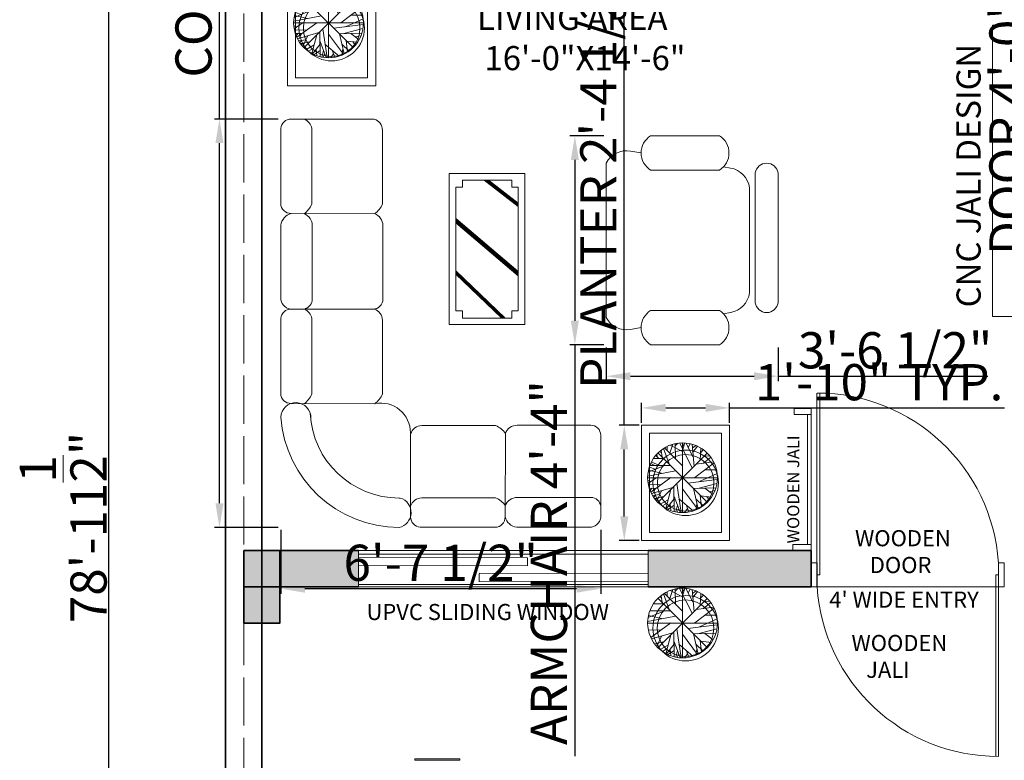
# Model space of a CAD drawing. Units: millimetres. Extents: x 595116 to 630915, y 909473 to 920225.
# Tile 118 of 134: x 629260 to 629505, y 919558 to 919742. Entities that reach past the tile are written whole.
import ezdxf

# ---------------------------------------------------------------- set-up
doc = ezdxf.new("R2010")
doc.units = ezdxf.units.MM
doc.linetypes.add('ACAD_ISO02W100', pattern=[15, 12, -3])
for name, color, linetype, lineweight in [('A-AREA-IDEN', 7, 'Continuous', 20), ('A-FLOR-SCRN', 31, 'Continuous', 18), ('A-FURN', 32, 'Continuous', 18), ('A-WALL', 1, 'Continuous', 35), ('A-WALL-PATT', 8, 'Continuous', 13), ('C-PRKG-VEHI', 8, 'Continuous', 13), ('C-PROP-REF', 240, 'ACAD_ISO02W100', 13), ('Column', 6, 'Continuous', 35), ('Dimension', 3, 'Continuous', 18), ('Doors', 31, 'Continuous', 20), ('L-PLNT', 85, 'Continuous', 13), ('Text', 7, 'Continuous', 18), ('Windows', 33, 'Continuous', 18)]:
    doc.layers.add(name, color=color, linetype=linetype, lineweight=lineweight)
doc.styles.get("Standard").update_dxf_attribs({"font": 'arial.ttf'})
doc.dimstyles.new('ISO-25', dxfattribs={"dimtxt": 9, "dimasz": 6, "dimexe": 1.25, "dimexo": 0.625, "dimtad": 1, "dimlunit": 4, "dimtxsty": 'Standard', "dimcen": 2.5, "dimadec": 0, "dimazin": 0, "dimtfac": 1, "dimtmove": 0, "dimatfit": 3, "dimfxl": 1, "dimarcsym": 0})

# ---------------------------------------------------------------- blocks, each defined once
blk = doc.blocks.new('KWD')
for points in [[(629753.63, 919957.93), (629752.54, 919957.93), (629752.54, 919953.43), (629753.63, 919953.43)], [(629787.45, 919957.93), (629787.45, 919953.43), (629788.54, 919953.43), (629788.54, 919957.93)]]:
    blk.add_lwpolyline(points, close=True)
blk.add_lwpolyline([(629753.63, 919921.79), (629753.63, 919955.68), (629754.13, 919955.68), (629754.13, 919921.8)])
blk.add_arc((629753.64, 919955.68), 33.88, 269.99, 356.196)
blk = doc.blocks.new('A$C2F471D6A')
for p, q in [((2695.9, 2657.3), (2692.2, 1939.9)), ((1797.2, 841.3), (2182.6, 1242.6)), ((1797.2, 833.9), (2189.8, 1242.6)), ((1797.2, 826.4), (2197, 1242.6)), ((1797.2, 818.9), (2204.2, 1242.6)), ((1797.2, 848.8), (2175.4, 1242.6)), ((2161.4, 709.9), (2615.3, 1243.3)), ((2168.6, 709.9), (2622.5, 1243.3)), ((2175.8, 709.9), (2629.7, 1243.3)), ((2183, 709.9), (2636.9, 1243.3)), ((2190.2, 709.9), (2644.1, 1243.3)), ((2197.4, 709.9), (2651.3, 1243.3)), ((2755.3, 709.9), (2980.5, 1000.5)), ((2762.5, 709.9), (2981.1, 992)), ((2769.7, 709.9), (2981.1, 982.7)), ((2776.9, 709.9), (2981.1, 973.4)), ((2784.1, 709.9), (2981.1, 964.1)), ((807.3, 817.6), (89.9, 821.3))]:
    blk.add_line(p, q)
for points in [[(0, 1730, -0.393715), (947.4, 2744.8)], [(946.9, 2744.9, -1), (937.9, 2487, 1)], [(1060.8, 1939.9, 0.132391), (1145.9, 1873.4), (1778.5, 1873.4, 0.326313), (1874.7, 1943.6), (1874.7, 2657.3, 0.389129), (1793.3, 2746), (1149.6, 2746, 0.426582), (1064.5, 2657.3, 0.287811)], [(1060.8, 2545.7, 0.132391), (1145.9, 2479.2), (1778.5, 2479.2, 0.287096), (1869.3, 2536)], [(1878.2, 2536, 0.331063), (1959.6, 2475.5), (2433.2, 2475.5)], [(2433.2, 2475.5), (2592.3, 2475.5, 0.316456), (2692.2, 2545.7, 0.132391), (2777.2, 2479.2), (3409.9, 2479.2, 0.287096), (3500.7, 2536)], [(252.5, 1720.4), (252.5, 1729.1, -0.399385), (979.3, 2493.9)], [(812.9, 1633.4, 0.469502), (1063.7, 1935.5, -1.204519)], [(252.5, 1720.4, -0.77294), (0, 1730, -1)], [(257.4, 558.6), (257.4, 717.7, 0.316456), (187.2, 817.6, 0.132391), (253.7, 902.7), (253.7, 1535.3, 0.326313), (183.5, 1631.5), (180.9, 1631.5, 0.389129)], [(180.9, 0.4, 0.385191), (257.4, 85.1), (257.4, 558.6)]]:
    blk.add_lwpolyline(points, format="xyb")
for points in [[(2433.2, 1869.7), (2592.3, 1869.7, 0.316456), (2692.2, 1939.9, 0.132391), (2777.2, 1873.4), (3409.9, 1873.4, 0.326313), (3506.1, 1943.6), (3506.1, 2657.3, 0.389129), (3424.7, 2746), (2780.9, 2746, 0.426582), (2695.9, 2657.3, 0.287811), (2596, 2746), (1970.7, 2746, 0.366167), (1874.5, 2664.7), (1874.5, 1954.7, 0.414362), (1959.6, 1869.7)], [(877.5, 558.6), (877.5, 717.7, 0.316456), (807.3, 817.6, 0.132391), (873.8, 902.7), (873.8, 1535.3, 0.326313), (803.6, 1631.5), (89.9, 1631.5, 0.389129), (1.2, 1550.1), (1.2, 906.4, 0.426582), (89.9, 821.3, 0.287811), (1.2, 721.4), (1.2, 96.2, 0.366167), (82.5, 0), (792.5, 0, 0.414362), (877.5, 85.1)]]:
    blk.add_lwpolyline(points, format="xyb", close=True)
blk.add_lwpolyline([(1064.5, 2657.3), (1060.8, 1939.9)])
for points in [[(1742.1, 652.3), (1742.1, 1300.3), (3038.1, 1300.3), (3038.1, 652.3)], [(2981.1, 1185.5), (2920, 1185.5), (2920, 1242.6), (1860.2, 1242.6), (1860.2, 1185.5), (1797.2, 1185.5), (1797.2, 762.2), (1860.2, 762.2), (1860.2, 709.1), (2920, 709.1), (2920, 762.2), (2981.1, 762.2)]]:
    blk.add_lwpolyline(points, close=True)
blk = doc.blocks.new('A$C20666D62')
for p, q in [((444.1, 457.2), (99.1, 457.2)), ((444.1, 396.2), (99.1, 396.2)), ((418, 381), (138.3, 381)), ((82.7, 311.8), (86, 330.2)), ((473.6, 311.8), (470.3, 330.2)), ((0, 118.1), (0, 301)), ((91.4, 301), (91.4, 118.1)), ((464.9, 301), (464.9, 118.1)), ((556.2, 118.1), (556.2, 301)), ((45.7, 92.8), (41.2, 64.6)), ((510.5, 92.8), (515.1, 64.6)), ((72.9, 0), (483.4, 0))]:
    blk.add_line(p, q)
for centre, radius, start, end in [((103.7, 426.7), 30.8, 98.7722, 261.228), ((439.5, 426.7), 30.8, 278.771, 81.2286), ((146.7, 320), 61.6, 97.9219, 170.441), ((409.6, 320), 61.6, 9.5598, 82.0778), ((45.7, 272.6), 53.9, 31.8953, 148.105), ((510.5, 272.6), 53.9, 31.8953, 148.105), ((45.7, 146.6), 53.8, 211.888, 328.112), ((510.5, 146.6), 53.8, 211.888, 328.112), ((98.9, 52.9), 58.9, 168.447, 243.852), ((457.4, 52.9), 58.9, 296.148, 11.5527)]:
    blk.add_arc(centre, radius, start, end)
blk = doc.blocks.new('A$C7ADB3080')
for p, q in [((0, 1141.1), (0, 1143.7)), ((0, 1143.7), (10.2, 1143.5)), ((0, 1136.6), (0, 1141.1)), ((0, 1131), (0, 1136.6)), ((0, 821.3), (0, 1131)), ((10.2, 1143.5), (10.2, 1140.7)), ((10.2, 1140.9), (10.2, 1143.5)), ((10.2, 1136.4), (10.2, 1140.9)), ((10.2, 1140.7), (10.2, 1136)), ((10.2, 1131.1), (10.2, 1136.4)), ((10.2, 1136), (10.2, 1130.9)), ((10.2, 821.4), (10.2, 1131.1)), ((10.2, 1130.9), (10.2, 821.4)), ((0, 816.5), (0, 821.3)), ((0, 812), (0, 816.5)), ((0, 808.8), (0, 812)), ((0, 808.8), (10.2, 808.8)), ((0, 808.8), (10.2, 808.7)), ((10.2, 816.5), (10.2, 821.4)), ((10.2, 821.4), (10.2, 816)), ((10.2, 811.8), (10.2, 816.5)), ((10.2, 816), (10.2, 811.6)), ((10.2, 808.8), (10.2, 811.8)), ((10.2, 811.6), (10.2, 808.7)), ((10.2, 808.7), (10.2, 808.8))]:
    blk.add_line(p, q)
blk = doc.blocks.new('*D128')
at = {"layer": 'Defpoints', "color": 0, "transparency": 16777216}
for p in [(629311.54, 920089.43), (629282.4, 919141.93), (629311.54, 919141.93)]:
    blk.add_point(p, dxfattribs=at)
at = {"layer": 'Dimension', "color": 0, "lineweight": -2, "transparency": 16777216}
for p, q in [((629310.92, 920089.43), (629281.15, 920089.43)), ((629282.4, 920083.43), (629282.4, 919147.93)), ((629310.92, 919141.93), (629281.15, 919141.93))]:
    blk.add_line(p, q, dxfattribs=at)
at = {"layer": 'Dimension', "color": 0, "transparency": 16777216}
for points in [[(629281.4, 920083.43), (629283.4, 920083.43), (629282.4, 920089.43)], [(629281.4, 919147.93), (629283.4, 919147.93), (629282.4, 919141.93)]]:
    blk.add_solid(points, dxfattribs=at)
at = {"layer": 'Dimension', "color": 0, "transparency": 16777216, "insert": (629271.16, 919615.68), "char_height": 9, "attachment_point": 5, "rotation": 90}
blk.add_mtext('78\'-11{\\H1x;\\S1/2;}"', dxfattribs=at)
blk = doc.blocks.new('POTTED-PLANT')
for p, q in [((4.85, 16.17), (4.88, 17.22)), ((5.49, 15.52), (6.28, 17.77)), ((5.61, 17.51), (8.67, 15.94)), ((6.86, 17.38), (7.52, 18.03)), ((6.89, 14.08), (6.86, 17.93)), ((7.9, 18.06), (11.06, 11.86)), ((9.02, 17.38), (8.46, 18.1)), ((8.67, 18.11), (8.67, 0.76)), ((8.74, 16.47), (9.2, 18.06)), ((11.32, 14.57), (9.46, 18.06)), ((10.09, 16.89), (10.53, 17.9)), ((11.52, 12.26), (11.04, 17.77)), ((11.14, 16.82), (12.03, 17.41)), ((11.24, 15.75), (12.36, 17.28)), ((14.75, 15.51), (2.6, 3.36)), ((14.75, 3.36), (2.6, 15.51)), ((2.87, 15.88), (3.4, 15.68)), ((3.32, 16.24), (3.58, 14.57)), ((3.96, 16.73), (5.31, 12.84)), ((4.16, 16.82), (8.64, 12.35)), ((13.25, 16.79), (13.05, 13.86)), ((13.17, 15.58), (13.86, 16.4)), ((14.04, 14.8), (15.41, 14.87)), ((4.01, 12.42), (0.12, 10.79)), ((0.57, 12.45), (5.66, 12.45)), ((1.47, 14.18), (3.93, 14.18)), ((16.53, 13.1), (11.7, 9.48)), ((12.05, 12.81), (16.38, 13.4)), ((13.91, 13.07), (15.74, 14.51)), ((0.04, 9.84), (6.94, 11.18)), ((0.19, 11.28), (3.48, 10.53)), ((12.92, 8.47), (17.27, 10.46)), ((14.24, 11.38), (17.09, 11.41)), ((0, 9.44), (17.35, 9.44)), ((0.22, 7.66), (3.4, 7.75)), ((0.78, 5.86), (5.74, 9.45)), ((7.22, 7.98), (8.31, 0.8)), ((10.02, 8.11), (17.3, 9.03)), ((12.49, 6.77), (17.19, 8.01)), ((0.98, 5.47), (6.25, 7.04)), ((3.48, 6.19), (2.31, 3.58)), ((5.79, 6.51), (4.54, 1.82)), ((6.53, 7.26), (6.56, 1.1)), ((8.67, 6.68), (12.41, 1.65)), ((11.37, 6.74), (12.54, 1.72)), ((11.39, 6.74), (16.97, 6.94)), ((13.07, 5.08), (13.35, 2.21)), ((13.22, 4.91), (15.85, 4.62)), ((14.19, 6.81), (16.25, 5.24)), ((3.99, 4.75), (1.72, 4.29)), ((5.1, 3.97), (3.07, 2.83)), ((4.88, 3.09), (3.65, 2.4)), ((6.56, 4.2), (4.67, 1.78)), ((6.56, 2.6), (5.05, 1.59)), ((5.56, 2.86), (5.79, 1.33)), ((6.56, 4.78), (8.11, 0.84)), ((7.45, 2.57), (7.01, 0.97)), ((7.78, 4.2), (11.26, 1.2)), ((9.53, 2.7), (10.2, 0.97)), ((11.98, 4.16), (13.78, 2.43)), ((12.26, 2.96), (12, 1.49)), ((7.75, 1.82), (7.32, 0.93)), ((9.89, 1.75), (9.23, 0.84))]:
    blk.add_line(p, q)
for centre, radius in [((8.67, 9.44), 8.67), ((9.43, 8.14), 8.14), ((9.43, 8.14), 7.03)]:
    blk.add_circle(centre, radius)
blk = doc.blocks.new('PLANTER-RECT')
for p, q in [((4.38, 22.08), (4.91, 21.89)), ((4.83, 22.44), (5.09, 20.78)), ((5.47, 22.93), (6.82, 19.05)), ((5.67, 23.03), (10.15, 18.56)), ((6.36, 22.38), (6.39, 23.42)), ((7, 21.72), (7.79, 23.98)), ((7.12, 23.71), (10.18, 22.15)), ((8.37, 23.58), (9.03, 24.24)), ((8.4, 20.29), (8.37, 24.14)), ((9.42, 24.27), (12.57, 18.07)), ((10.54, 23.58), (9.98, 24.3)), ((10.18, 24.32), (10.18, 6.97)), ((10.26, 22.67), (10.71, 24.27)), ((12.83, 20.78), (10.97, 24.27)), ((11.6, 23.09), (12.04, 24.11)), ((13.03, 18.46), (12.55, 23.98)), ((12.65, 23.03), (13.54, 23.62)), ((12.75, 21.95), (13.87, 23.49)), ((14.76, 23), (14.56, 20.06)), ((14.68, 21.79), (15.37, 22.61)), ((2.49, 19.6), (4.38, 18.66)), ((2.98, 20.39), (5.45, 20.39)), ((3.56, 21.17), (4.33, 20.42)), ((3.84, 20.91), (3.77, 21.46)), ((16.26, 21.71), (4.11, 9.57)), ((16.26, 9.57), (4.11, 21.71)), ((13.56, 19.02), (17.89, 19.6)), ((15.42, 19.28), (17.25, 20.71)), ((15.55, 21.01), (16.92, 21.07)), ((1.55, 16.05), (8.45, 17.38)), ((5.52, 18.62), (1.63, 16.99)), ((1.7, 17.48), (4.99, 16.73)), ((1.93, 18.23), (3.38, 17.78)), ((2.09, 18.66), (7.18, 18.66)), ((2.26, 19.18), (3.28, 18.69)), ((18.04, 19.31), (13.21, 15.69)), ((15.75, 17.58), (18.6, 17.61)), ((1.51, 15.64), (18.86, 15.64)), ((1.55, 14.94), (2.34, 14.68)), ((3.64, 15.62), (1.65, 14.19)), ((2.29, 12.07), (7.25, 15.66)), ((11.53, 14.32), (18.81, 15.23)), ((14.43, 14.68), (18.78, 16.67)), ((1.73, 13.86), (4.91, 13.96)), ((1.93, 12.98), (3.64, 13.05)), ((2.57, 13.01), (2.16, 12.46)), ((2.49, 11.67), (7.76, 13.24)), ((3.36, 12.85), (2.93, 11.84)), ((4.99, 12.39), (3.82, 9.78)), ((7.3, 12.72), (6.06, 8.02)), ((8.04, 13.47), (8.07, 7.3)), ((8.73, 14.19), (9.82, 7.01)), ((10.18, 12.88), (13.92, 7.86)), ((12.88, 12.95), (14.05, 7.92)), ((12.9, 12.95), (18.48, 13.14)), ((14, 12.98), (18.71, 14.22)), ((15.7, 13.01), (17.76, 11.45)), ((16.82, 12.16), (18.22, 12.43)), ((4.55, 11.45), (2.75, 11.22)), ((3.46, 11.28), (3.03, 10.79)), ((5.5, 10.96), (3.23, 10.5)), ((3.87, 10.63), (3.43, 10.24)), ((6.62, 10.17), (4.58, 9.03)), ((8.07, 10.4), (6.18, 7.99)), ((8.07, 10.99), (9.62, 7.04)), ((9.29, 10.4), (12.78, 7.4)), ((13.49, 10.37), (15.29, 8.64)), ((14.58, 11.28), (14.86, 8.41)), ((14.73, 11.12), (17.36, 10.83)), ((16.19, 10.92), (16.85, 10.14)), ((6.39, 9.29), (5.17, 8.61)), ((8.07, 8.8), (6.57, 7.79)), ((7.07, 9.06), (7.3, 7.53)), ((8.96, 8.77), (8.52, 7.17)), ((9.26, 8.02), (8.83, 7.14)), ((11.4, 7.96), (10.74, 7.04)), ((11.04, 8.9), (11.71, 7.17)), ((13.77, 9.16), (13.51, 7.69))]:
    blk.add_line(p, q)
for points in [[(0, 28.69), (21.89, 28.69), (21.89, 0), (0, 0)], [(2, 26.69), (19.89, 26.69), (19.89, 2), (2, 2)]]:
    blk.add_lwpolyline(points, close=True)
for centre, radius in [((10.18, 15.64), 8.67), ((10.95, 14.35), 8.14), ((10.95, 14.35), 7.03)]:
    blk.add_circle(centre, radius)
blk = doc.blocks.new('DOOR-ENTRY-SCREEN')
blk.add_lwpolyline([(45.09, 0), (45.09, 45.18), (44.42, 45.18), (44.42, 0.01)])
blk.add_arc((45.08, 45.18), 45.18, 183.804, 270.01)
blk = doc.blocks.new('COLUMN-RECT-9X18')
h = blk.add_hatch(color=256)
h.dxf.hatch_style = 1
h.paths.add_polyline_path([(9, 18), (0, 18), (0, 0), (9, 0)])
blk.add_lwpolyline([(0, 18), (9, 18), (9, 0), (0, 0)], close=True)
blk = doc.blocks.new('*D162')
at = {"layer": 'Defpoints', "color": 0, "transparency": 16777216}
for p in [(629505.04, 919832.11), (629505.04, 919783.93), (629512.27, 919783.93)]:
    blk.add_point(p, dxfattribs=at)
at = {"layer": 'Dimension', "color": 0, "lineweight": -2, "transparency": 16777216}
for p, q in [((629505.67, 919832.11), (629513.52, 919832.11)), ((629512.27, 919826.11), (629512.27, 919789.93)), ((629505.67, 919783.93), (629513.52, 919783.93)), ((629512.27, 919783.93), (629512.27, 919681.05))]:
    blk.add_line(p, q, dxfattribs=at)
at = {"layer": 'Dimension', "color": 0, "transparency": 16777216}
for points in [[(629511.27, 919826.11), (629513.27, 919826.11), (629512.27, 919832.11)], [(629511.27, 919789.93), (629513.27, 919789.93), (629512.27, 919783.93)]]:
    blk.add_solid(points, dxfattribs=at)
at = {"layer": 'Dimension', "color": 0, "transparency": 16777216, "insert": (629506.99, 919729.49), "char_height": 9, "attachment_point": 5, "rotation": 90}
blk.add_mtext('DOOR 4\'-0" TYP.', dxfattribs=at)
blk = doc.blocks.new('*D188')
at = {"layer": 'Defpoints', "color": 0, "transparency": 16777216}
for p in [(629410.6, 919641.11), (629414.9, 919641.11), (629414.9, 919612.42)]:
    blk.add_point(p, dxfattribs=at)
at = {"layer": 'Dimension', "color": 0, "lineweight": -2, "transparency": 16777216}
for p, q in [((629410.6, 919641.11), (629410.6, 919785.23)), ((629414.27, 919641.11), (629409.35, 919641.11)), ((629410.6, 919618.42), (629410.6, 919635.11)), ((629414.27, 919612.42), (629409.35, 919612.42))]:
    blk.add_line(p, q, dxfattribs=at)
at = {"layer": 'Dimension', "color": 0, "transparency": 16777216}
for points in [[(629409.6, 919635.11), (629411.6, 919635.11), (629410.6, 919641.11)], [(629409.6, 919618.42), (629411.6, 919618.42), (629410.6, 919612.42)]]:
    blk.add_solid(points, dxfattribs=at)
at = {"layer": 'Dimension', "color": 0, "transparency": 16777216, "insert": (629405.32, 919716.17), "char_height": 9, "attachment_point": 5, "rotation": 90}
blk.add_mtext('PLANTER 2\'-4 1/2" TYP.', dxfattribs=at)
blk = doc.blocks.new('*D189')
at = {"layer": 'Defpoints', "color": 0, "transparency": 16777216}
for p in [(629436.79, 919645.42), (629414.9, 919641.11), (629436.79, 919641.11)]:
    blk.add_point(p, dxfattribs=at)
at = {"layer": 'Dimension', "color": 0, "lineweight": -2, "transparency": 16777216}
for p, q in [((629414.9, 919641.74), (629414.9, 919646.67)), ((629436.79, 919641.74), (629436.79, 919646.67)), ((629420.9, 919645.42), (629430.79, 919645.42)), ((629436.79, 919645.42), (629505.05, 919645.42))]:
    blk.add_line(p, q, dxfattribs=at)
at = {"layer": 'Dimension', "color": 0, "transparency": 16777216}
for points in [[(629420.9, 919646.42), (629420.9, 919644.42), (629414.9, 919645.42)], [(629430.79, 919646.42), (629430.79, 919644.42), (629436.79, 919645.42)]]:
    blk.add_solid(points, dxfattribs=at)
at = {"layer": 'Dimension', "color": 0, "transparency": 16777216, "insert": (629473.92, 919650.64), "char_height": 9, "attachment_point": 5}
blk.add_mtext('1\'-10" TYP.', dxfattribs=at)
blk = doc.blocks.new('*D202')
at = {"layer": 'Defpoints', "color": 0, "transparency": 16777216}
for p in [(629310, 919717.23), (629325.23, 919717.23), (629325.23, 919615.7)]:
    blk.add_point(p, dxfattribs=at)
at = {"layer": 'Dimension', "color": 0, "lineweight": -2, "transparency": 16777216}
for p, q in [((629310, 919717.23), (629310, 919864.97)), ((629324.61, 919717.23), (629308.75, 919717.23)), ((629310, 919621.7), (629310, 919711.23)), ((629324.61, 919615.7), (629308.75, 919615.7))]:
    blk.add_line(p, q, dxfattribs=at)
at = {"layer": 'Dimension', "color": 0, "transparency": 16777216}
for points in [[(629309, 919711.23), (629311, 919711.23), (629310, 919717.23)], [(629309, 919621.7), (629311, 919621.7), (629310, 919615.7)]]:
    blk.add_solid(points, dxfattribs=at)
at = {"layer": 'Dimension', "color": 0, "transparency": 16777216, "insert": (629304.72, 919794.1), "char_height": 9, "attachment_point": 5, "rotation": 90}
blk.add_mtext('CORNER SOFA 8\'-5 1/2"', dxfattribs=at)
blk = doc.blocks.new('*D203')
at = {"layer": 'Defpoints', "color": 0, "transparency": 16777216}
for p in [(629325.23, 919615.7), (629404.75, 919615.7), (629325.23, 919600.47)]:
    blk.add_point(p, dxfattribs=at)
at = {"layer": 'Dimension', "color": 0, "lineweight": -2, "transparency": 16777216}
for p, q in [((629325.23, 919615.07), (629325.23, 919599.22)), ((629404.75, 919615.07), (629404.75, 919599.22)), ((629398.75, 919600.47), (629331.23, 919600.47))]:
    blk.add_line(p, q, dxfattribs=at)
at = {"layer": 'Dimension', "color": 0, "transparency": 16777216}
for points in [[(629331.23, 919601.47), (629331.23, 919599.47), (629325.23, 919600.47)], [(629398.75, 919601.47), (629398.75, 919599.47), (629404.75, 919600.47)]]:
    blk.add_solid(points, dxfattribs=at)
at = {"layer": 'Dimension', "color": 0, "transparency": 16777216, "insert": (629364.99, 919605.74), "char_height": 9, "attachment_point": 5}
blk.add_mtext('6\'-7 1/2"', dxfattribs=at)
blk = doc.blocks.new('*D204')
at = {"layer": 'Defpoints', "color": 0, "transparency": 16777216}
for p in [(629406.11, 919713.07), (629398.32, 919661.09), (629406.11, 919661.09)]:
    blk.add_point(p, dxfattribs=at)
at = {"layer": 'Dimension', "color": 0, "lineweight": -2, "transparency": 16777216}
for p, q in [((629405.49, 919713.07), (629397.07, 919713.07)), ((629398.32, 919707.07), (629398.32, 919667.09)), ((629405.49, 919661.09), (629397.07, 919661.09)), ((629398.32, 919661.09), (629398.32, 919558.84))]:
    blk.add_line(p, q, dxfattribs=at)
at = {"layer": 'Dimension', "color": 0, "transparency": 16777216}
for points in [[(629397.32, 919707.07), (629399.32, 919707.07), (629398.32, 919713.07)], [(629397.32, 919667.09), (629399.32, 919667.09), (629398.32, 919661.09)]]:
    blk.add_solid(points, dxfattribs=at)
at = {"layer": 'Dimension', "color": 0, "transparency": 16777216, "insert": (629393.04, 919606.96), "char_height": 9, "attachment_point": 5, "rotation": 90}
blk.add_mtext('ARMCHAIR 4\'-4"', dxfattribs=at)
blk = doc.blocks.new('*D205')
at = {"layer": 'Defpoints', "color": 0, "transparency": 16777216}
for p in [(629406.11, 919661.09), (629448.84, 919661.09), (629448.84, 919653.29)]:
    blk.add_point(p, dxfattribs=at)
at = {"layer": 'Dimension', "color": 0, "lineweight": -2, "transparency": 16777216}
for p, q in [((629406.11, 919660.46), (629406.11, 919652.04)), ((629448.84, 919660.46), (629448.84, 919652.04)), ((629412.11, 919653.29), (629442.84, 919653.29)), ((629448.84, 919653.29), (629500.98, 919653.29))]:
    blk.add_line(p, q, dxfattribs=at)
at = {"layer": 'Dimension', "color": 0, "transparency": 16777216}
for points in [[(629412.11, 919654.29), (629412.11, 919652.29), (629406.11, 919653.29)], [(629442.84, 919654.29), (629442.84, 919652.29), (629448.84, 919653.29)]]:
    blk.add_solid(points, dxfattribs=at)
at = {"layer": 'Dimension', "color": 0, "transparency": 16777216, "insert": (629477.91, 919658.57), "char_height": 9, "attachment_point": 5}
blk.add_mtext('3\'-6 1/2"', dxfattribs=at)

msp = doc.modelspace()

# ---------------------------------------------------------------- hatches: boundary and pattern name
at = {"layer": 'A-WALL-PATT'}
h = msp.add_hatch(color=256, dxfattribs=at)
h.dxf.hatch_style = 1
h.paths.add_polyline_path([(629344.541, 919609.928), (629325.041, 919609.928), (629325.041, 919600.928), (629344.541, 919600.928)])
h = msp.add_hatch(color=256, dxfattribs=at)
h.dxf.hatch_style = 1
h.paths.add_polyline_path([(629457.041, 919606.928), (629457.041, 919609.928), (629452.524, 919609.928), (629416.541, 919609.928), (629416.541, 919600.928), (629457.041, 919600.928)])

# ---------------------------------------------------------------- linework, layer by layer
at = {"layer": 'A-FLOR-SCRN'}
for p, q in [((629456.126, 919643.743), (629456.126, 919611.433)), ((629457.041, 919611.433), (629457.041, 919643.743))]:
    msp.add_line(p, q, dxfattribs=at)
for points in [[(629502.1, 919740.57), (629509.588, 919740.57), (629509.588, 919668.119), (629502.1, 919668.119)], [(629457.041, 919645.249), (629452.806, 919645.249), (629452.806, 919643.743), (629457.041, 919643.743)], [(629457.041, 919609.928), (629452.524, 919609.928), (629452.524, 919611.433), (629457.041, 919611.433)]]:
    msp.add_lwpolyline(points, close=True, dxfattribs=at)
at = {"layer": 'A-WALL'}
for p, q in [((629320.541, 919345.928), (629320.541, 919957.928)), ((629316.041, 919609.928), (629344.541, 919609.928)), ((629416.541, 919609.928), (629457.041, 919609.928)), ((629457.041, 919609.928), (629457.041, 919600.928)), ((629316.041, 919600.928), (629344.541, 919600.928)), ((629416.541, 919600.928), (629457.041, 919600.928))]:
    msp.add_line(p, q, dxfattribs=at)
msp.add_lwpolyline([(629311.541, 919345.928), (629311.541, 919957.928)], dxfattribs=at)
at = {"layer": 'C-PROP-REF'}
msp.add_line((629316.041, 919146.428), (629316.041, 920084.928), dxfattribs=at)
at = {"layer": 'Doors'}
msp.add_line((629458.498, 919600.928), (629503.583, 919600.928), dxfattribs=at)
msp.add_lwpolyline([(629458.498, 919606.928), (629458.498, 919600.928), (629457.041, 919600.928), (629457.041, 919606.928)], close=True, dxfattribs=at)
at = {"layer": 'Windows'}
for p, q in [((629344.541, 919600.928), (629344.541, 919609.928)), ((629344.541, 919609.928), (629416.541, 919609.928)), ((629416.541, 919600.928), (629416.541, 919609.928)), ((629344.547, 919608.211), (629386.541, 919608.126)), ((629386.541, 919608.126), (629386.541, 919606.126)), ((629344.543, 919606.211), (629386.541, 919606.126)), ((629374.541, 919604.346), (629416.539, 919604.26)), ((629374.541, 919604.15), (629374.541, 919602.15)), ((629374.541, 919602.346), (629416.535, 919602.26)), ((629344.541, 919600.928), (629416.541, 919600.928))]:
    msp.add_line(p, q, dxfattribs=at)
msp.add_lwpolyline([(629344.541, 919609.023), (629416.541, 919609.023), (629416.541, 919601.497), (629344.541, 919601.497)], close=True, dxfattribs=at)

# ---------------------------------------------------------------- block references
at = {"layer": 'A-FURN'}
for name, p, xscale, yscale, zscale, rotation in [('A$C2F471D6A', (629404.753, 919615.695), 0.0289589963073228, 0.0289589963073228, 0.0289589963073228, 90), ('A$C20666D62', (629406.114, 919713.069), 0.0934465932983005, 0.0934465932983005, 0.0934465932983005, 270)]:
    msp.add_blockref(name, p, dxfattribs=dict(at, xscale=xscale, yscale=yscale, zscale=zscale, rotation=rotation))
at = {"layer": 'C-PRKG-VEHI', "xscale": 0.0334614614063694, "yscale": 0.0334614614063694, "zscale": 0.0334614614063694, "rotation": 270}
msp.add_blockref('A$C7ADB3080', (629331.465, 919558.166), dxfattribs=at)
at = {"layer": 'Column'}
msp.add_blockref('COLUMN-RECT-9X18', (629316.041, 919591.928), dxfattribs=at)
at = {"layer": 'Doors', "xscale": -1.333333333333333, "yscale": 1.333333333333333, "zscale": 1.333333333333333, "rotation": 180}
msp.add_blockref('KWD', (-210213.014, 2146211.498), dxfattribs=at)
at = {"layer": 'Doors'}
msp.add_blockref('DOOR-ENTRY-SCREEN', (629458.498, 919558.748), dxfattribs=at)
at = {"layer": 'L-PLNT'}
for name, p in [('PLANTER-RECT', (629326.929, 919725.477)), ('PLANTER-RECT', (629414.899, 919612.422)), ('POTTED-PLANT', (629416.41, 919582.492))]:
    msp.add_blockref(name, p, dxfattribs=at)

# ---------------------------------------------------------------- texts
at = {"layer": 'A-AREA-IDEN', "insert": (629370.361, 919745.376), "char_height": 6, "attachment_point": 1}
msp.add_mtext_dynamic_manual_height_columns('{  LIVING AREA\\P   16\'-0"X14\'-6"}', width=83.57324, gutter_width=12.5, heights=[0], dxfattribs=at)
at = {"layer": 'Text', "attachment_point": 1, "rotation": 90}
for s, width, insert, char_height in [('{CNC JALI DESIGN}', 83.57324, (629493.158, 919670.402), 6), ('{     WOODEN JALI}', 61.33456, (629451.088, 919607.128), 3)]:
    msp.add_mtext_dynamic_manual_height_columns(s, width=width, gutter_width=12.5, heights=[0], dxfattribs=dict(at, insert=insert, char_height=char_height))
at = {"layer": 'Text', "char_height": 4, "attachment_point": 1}
for s, width, insert in [('{     WOODEN\\P        DOOR}', 61.33456, (629461.833, 919615.018)), ("{4' WIDE ENTRY}", 61.33456, (629461.554, 919599.749)), ('{ UPVC SLIDING WINDOW}', 72.55106, (629345.324, 919596.673)), ('{     WOODEN\\P        JALI}', 61.33456, (629460.946, 919588.969))]:
    msp.add_mtext_dynamic_manual_height_columns(s, width=width, gutter_width=12.5, heights=[0], dxfattribs=dict(at, insert=insert))

# ---------------------------------------------------------------- dimensions: what is measured, and where the dimension line sits
at = {"layer": 'Dimension'}
for base, p1, p2, angle, override, picture, middle in [((629282.395, 919141.928), (629311.541, 920089.428), (629311.541, 919141.928), 90, {"dimclrd": 0, "dimclre": 0, "dimclrt": 0}, '*D128', (629271.157, 919615.678)), ((629325.23, 919600.466), (629404.753, 919615.695), (629325.23, 919615.695), 180, {"dimdec": 1, "dimlfac": 1, "dimrnd": 0, "dimzin": 1, "dimdsep": 46, "dimlunit": 4, "dimfrac": 2}, '*D203', (629364.992, 919605.744))]:
    dim = msp.add_linear_dim(base=base, p1=p1, p2=p2, angle=angle, dimstyle='ISO-25', override=override, dxfattribs=at)
    dim.commit()
    dim.dimension.update_dxf_attribs({"geometry": picture, "text_midpoint": middle})
for base, p1, p2, angle, text, picture, middle in [((629310.001, 919717.228), (629325.23, 919615.695), (629325.23, 919717.228), 90, 'CORNER SOFA <>', '*D202', (629304.719, 919794.1)), ((629512.268, 919783.928), (629505.041, 919832.112), (629505.041, 919783.928), 270, 'DOOR <> TYP.', '*D162', (629506.987, 919729.491)), ((629410.595, 919641.114), (629414.899, 919612.422), (629414.899, 919641.114), 90, 'PLANTER <> TYP.', '*D188', (629405.317, 919716.172)), ((629398.317, 919661.087), (629406.114, 919713.069), (629406.114, 919661.087), 270, 'ARMCHAIR <>', '*D204', (629393.039, 919606.964))]:
    dim = msp.add_linear_dim(base=base, p1=p1, p2=p2, angle=angle, text=text, dimstyle='ISO-25', override={"dimdec": 1, "dimlfac": 1, "dimrnd": 0, "dimzin": 1, "dimdsep": 46, "dimlunit": 4, "dimfrac": 2}, dxfattribs=at)
    dim.commit()
    dim.dimension.update_dxf_attribs({"geometry": picture, "text_midpoint": middle})
dim = msp.add_linear_dim(base=(629448.838, 919653.29), p1=(629406.114, 919661.087), p2=(629448.838, 919661.087), dimstyle='ISO-25', override={"dimdec": 1, "dimlfac": 1, "dimrnd": 0, "dimzin": 1, "dimdsep": 46, "dimlunit": 4, "dimfrac": 2}, dxfattribs=at)
dim.commit()
dim.dimension.update_dxf_attribs({"geometry": '*D205', "text_midpoint": (629477.908, 919658.572)})
dim = msp.add_linear_dim(base=(629436.791, 919645.418), p1=(629414.899, 919641.114), p2=(629436.791, 919641.114), text='<> TYP.', dimstyle='ISO-25', override={"dimdec": 1, "dimlfac": 1, "dimrnd": 0, "dimzin": 1, "dimdsep": 46, "dimlunit": 4, "dimfrac": 2}, dxfattribs=at)
dim.commit()
dim.dimension.update_dxf_attribs({"geometry": '*D189', "text_midpoint": (629473.918, 919650.638)})

doc.saveas('drawing.dxf')
